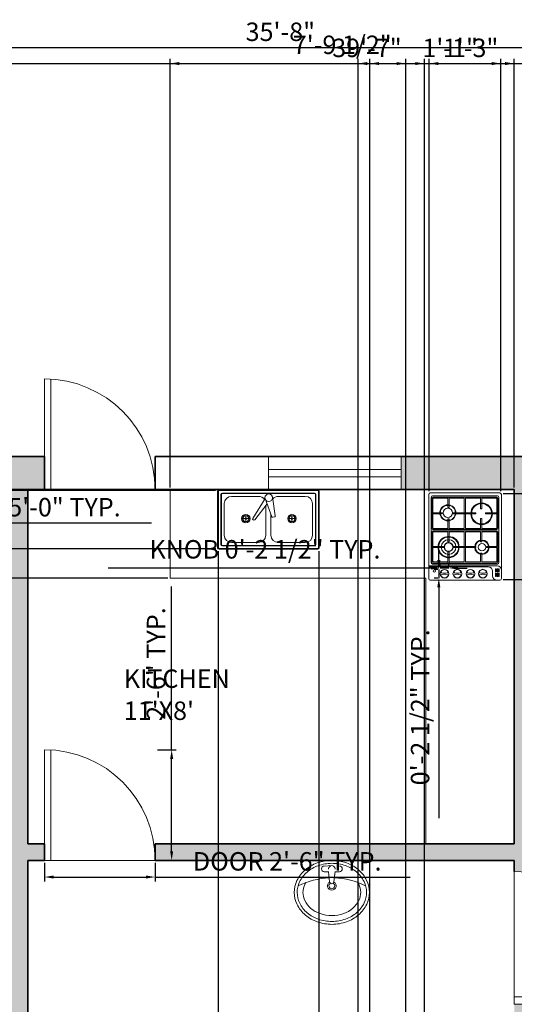
# Model space of a CAD drawing. Units: inches. Extents: x 2923 to 3500, y 1684 to 2381.
# Tile 11 of 12: x 3112 to 3247, y 2114 to 2381. Entities that reach past the tile are written whole.
import ezdxf

# ---------------------------------------------------------------- set-up
doc = ezdxf.new("R2010")
doc.units = ezdxf.units.IN
for name, color, linetype, lineweight in [('A-ANNO-DIMS', 2, 'Continuous', 18), ('A-AREA-IDEN', 7, 'Continuous', 18), ('A-DOOR', 3, 'Continuous', 18), ('A-EQPM', 8, 'Continuous', 18), ('A-FLOR-CASE', 7, 'Continuous', 20), ('A-FLOR-FIXT', 8, 'Continuous', 18), ('A-GLAZ', 4, 'Continuous', 18), ('A-WALL', 7, 'Continuous', 35), ('A-WALL-PATT', 9, 'Continuous', 13)]:
    doc.layers.add(name, color=color, linetype=linetype, lineweight=lineweight)
doc.styles.get("Standard").update_dxf_attribs({"font": 'txt', "height": 5})
doc.dimstyles.new('ISO-25', dxfattribs={"dimtxt": 5, "dimasz": 2.5, "dimexe": 1.25, "dimexo": 0.625, "dimtad": 1, "dimlunit": 3, "dimtxsty": 'Standard', "dimcen": 2.5, "dimadec": 0, "dimazin": 0, "dimtfac": 1, "dimtmove": 0, "dimatfit": 3, "dimfxl": 1, "dimarcsym": 0})

# ---------------------------------------------------------------- blocks, each defined once
blk = doc.blocks.new('*D2')
at = {"layer": 'A-ANNO-DIMS', "color": 0, "lineweight": -2, "transparency": 16777216}
for p, q in [((2969.23, 2263.03), (2969.23, 2374.52)), ((2971.73, 2373.27), (3394.73, 2373.27)), ((3397.23, 2263.03), (3397.23, 2374.52))]:
    blk.add_line(p, q, dxfattribs=at)
at = {"layer": 'A-ANNO-DIMS', "color": 0, "transparency": 16777216}
for points in [[(2971.73, 2373.69), (2971.73, 2372.86), (2969.23, 2373.27)], [(3394.73, 2373.69), (3394.73, 2372.86), (3397.23, 2373.27)]]:
    blk.add_solid(points, dxfattribs=at)
at = {"layer": 'Defpoints', "color": 0, "transparency": 16777216}
for p in [(3397.23, 2373.27), (2969.23, 2262.41), (3397.23, 2262.41)]:
    blk.add_point(p, dxfattribs=at)
at = {"layer": 'A-ANNO-DIMS', "color": 0, "transparency": 16777216, "insert": (3183.23, 2376.87), "char_height": 5, "attachment_point": 5}
blk.add_mtext('35\'-8"', dxfattribs=at)
blk = doc.blocks.new('DOOR-SINGLE-36IN')
for p, q in [((36, 36), (0, 36)), ((34, 0.06), (34, 36)), ((36, 0), (36, 36))]:
    blk.add_line(p, q)
blk.add_arc((36, 36), 36, 180, 270)
blk = doc.blocks.new('DOOR-SINGLE-30IN')
for p, q in [((0, 30), (0, 0)), ((1.67, 29.95), (1.67, 0)), ((0, 0), (30, 0))]:
    blk.add_line(p, q)
blk.add_arc((0, 0), 30, 0, 90)
blk = doc.blocks.new('WINDOW-36IN')
for p, q in [((36, 9), (0, 9)), ((0, 9), (0, 0)), ((36, 0), (36, 9)), ((36, 5.5), (0, 5.5)), ((36, 3.5), (0, 3.5)), ((0, 0), (36, 0))]:
    blk.add_line(p, q)
blk = doc.blocks.new('RANGE-CONTROL-KNOB')
blk.add_circle((1.19, 1.19), 1.19)
for centre, radius, start, end in [((0.4, 1.64), 0.197, 150.2471, 261.5797), ((0.4, 0.73), 0.197, 98.4203, 209.7529), ((1.19, 1.19), 1.11, 29.7529, 150.2471), ((1.19, 1.19), 1.11, 209.7529, 330.2471), ((1.19, 4.76), 3.42, 256.1268, 283.8732), ((1.19, -2.39), 3.42, 76.1268, 103.8732), ((1.98, 1.64), 0.197, 278.4203, 29.7529), ((1.98, 0.73), 0.197, 330.2471, 81.5797)]:
    blk.add_arc(centre, radius, start, end)
blk = doc.blocks.new('*D21')
at = {"layer": 'A-ANNO-DIMS', "color": 0, "lineweight": -2, "transparency": 16777216}
for p, q in [((3014.23, 2252.78), (3014.23, 2243.16)), ((3074.23, 2252.78), (3074.23, 2243.16)), ((3016.73, 2244.41), (3071.73, 2244.41)), ((3074.23, 2244.41), (3148.22, 2244.41))]:
    blk.add_line(p, q, dxfattribs=at)
at = {"layer": 'A-ANNO-DIMS', "color": 0, "transparency": 16777216}
for points in [[(3016.73, 2244.82), (3016.73, 2243.99), (3014.23, 2244.41)], [(3071.73, 2244.82), (3071.73, 2243.99), (3074.23, 2244.41)]]:
    blk.add_solid(points, dxfattribs=at)
at = {"layer": 'Defpoints', "color": 0, "transparency": 16777216}
for p in [(3014.23, 2253.41), (3074.23, 2253.41), (3074.23, 2244.41)]:
    blk.add_point(p, dxfattribs=at)
at = {"layer": 'A-ANNO-DIMS', "color": 0, "transparency": 16777216, "insert": (3112.47, 2248.01), "char_height": 5, "attachment_point": 5}
blk.add_mtext('SLIDER 5\'-0" TYP.', dxfattribs=at)
blk = doc.blocks.new('*D27')
at = {"layer": 'A-ANNO-DIMS', "color": 0, "lineweight": -2, "transparency": 16777216}
for p, q in [((3119.23, 2152.28), (3119.23, 2147.16)), ((3149.23, 2152.28), (3149.23, 2147.16)), ((3121.73, 2148.41), (3146.73, 2148.41)), ((3149.23, 2148.41), (3218.46, 2148.41))]:
    blk.add_line(p, q, dxfattribs=at)
at = {"layer": 'A-ANNO-DIMS', "color": 0, "transparency": 16777216}
for points in [[(3121.73, 2148.82), (3121.73, 2147.99), (3119.23, 2148.41)], [(3146.73, 2148.82), (3146.73, 2147.99), (3149.23, 2148.41)]]:
    blk.add_solid(points, dxfattribs=at)
at = {"layer": 'Defpoints', "color": 0, "transparency": 16777216}
for p in [(3119.23, 2152.91), (3149.23, 2152.91), (3149.23, 2148.41)]:
    blk.add_point(p, dxfattribs=at)
at = {"layer": 'A-ANNO-DIMS', "color": 0, "transparency": 16777216, "insert": (3185.09, 2152.01), "char_height": 5, "attachment_point": 5}
blk.add_mtext('DOOR 2\'-6" TYP.', dxfattribs=at)
blk = doc.blocks.new('*D28')
at = {"layer": 'A-ANNO-DIMS', "color": 0, "lineweight": -2, "transparency": 16777216}
for p, q in [((3153.73, 2182.91), (3153.73, 2227.13)), ((3149.85, 2182.91), (3154.98, 2182.91)), ((3153.73, 2155.41), (3153.73, 2180.41)), ((3149.85, 2152.91), (3154.98, 2152.91))]:
    blk.add_line(p, q, dxfattribs=at)
at = {"layer": 'A-ANNO-DIMS', "color": 0, "transparency": 16777216}
for points in [[(3153.31, 2180.41), (3154.15, 2180.41), (3153.73, 2182.91)], [(3153.31, 2155.41), (3154.15, 2155.41), (3153.73, 2152.91)]]:
    blk.add_solid(points, dxfattribs=at)
at = {"layer": 'Defpoints', "color": 0, "transparency": 16777216}
for p in [(3149.23, 2182.91), (3153.73, 2182.91), (3149.23, 2152.91)]:
    blk.add_point(p, dxfattribs=at)
at = {"layer": 'A-ANNO-DIMS', "color": 0, "transparency": 16777216, "insert": (3150.13, 2206.27), "char_height": 5, "attachment_point": 5, "rotation": 90}
blk.add_mtext('2\'-6" TYP.', dxfattribs=at)
blk = doc.blocks.new('*D43')
at = {"layer": 'A-ANNO-DIMS', "color": 0, "lineweight": -2, "transparency": 16777216}
for p, q in [((3224.09, 2232.16), (3136.53, 2232.16)), ((3226.59, 2232.43), (3226.59, 2233.41)), ((3228.96, 2232.16), (3226.59, 2232.16)), ((3228.96, 2232.43), (3228.96, 2233.41)), ((3231.46, 2232.16), (3233.96, 2232.16))]:
    blk.add_line(p, q, dxfattribs=at)
at = {"layer": 'A-ANNO-DIMS', "color": 0, "transparency": 16777216}
for points in [[(3224.09, 2232.58), (3224.09, 2231.74), (3226.59, 2232.16)], [(3231.46, 2232.58), (3231.46, 2231.74), (3228.96, 2232.16)]]:
    blk.add_solid(points, dxfattribs=at)
at = {"layer": 'Defpoints', "color": 0, "transparency": 16777216}
for p in [(3226.59, 2232.16), (3226.59, 2231.8), (3228.96, 2231.8)]:
    blk.add_point(p, dxfattribs=at)
at = {"layer": 'A-ANNO-DIMS', "color": 0, "transparency": 16777216, "insert": (3179.06, 2236.59), "char_height": 5, "attachment_point": 5}
blk.add_mtext('KNOB 0\'-2 1/2" TYP.', dxfattribs=at)
blk = doc.blocks.new('*D44')
at = {"layer": 'A-ANNO-DIMS', "color": 0, "lineweight": -2, "transparency": 16777216}
for p, q in [((3226.23, 2234.3), (3226.23, 2236.8)), ((3225.96, 2231.8), (3224.98, 2231.8)), ((3226.23, 2231.8), (3226.23, 2229.43)), ((3225.96, 2229.43), (3224.98, 2229.43)), ((3226.23, 2226.93), (3226.23, 2164.37))]:
    blk.add_line(p, q, dxfattribs=at)
at = {"layer": 'A-ANNO-DIMS', "color": 0, "transparency": 16777216}
for points in [[(3225.82, 2234.3), (3226.65, 2234.3), (3226.23, 2231.8)], [(3225.82, 2226.93), (3226.65, 2226.93), (3226.23, 2229.43)]]:
    blk.add_solid(points, dxfattribs=at)
at = {"layer": 'Defpoints', "color": 0, "transparency": 16777216}
for p in [(3226.59, 2231.8), (3226.23, 2229.43), (3226.59, 2229.43)]:
    blk.add_point(p, dxfattribs=at)
at = {"layer": 'A-ANNO-DIMS', "color": 0, "transparency": 16777216, "insert": (3221.8, 2194.4), "char_height": 5, "attachment_point": 5, "rotation": 90}
blk.add_mtext('0\'-2 1/2" TYP.', dxfattribs=at)
blk = doc.blocks.new('*D49')
at = {"layer": 'A-ANNO-DIMS', "color": 0, "lineweight": -2, "transparency": 16777216}
for p, q in [((2969.23, 2263.03), (2969.23, 2370.16)), ((3444.23, 2110.03), (3444.23, 2370.16)), ((2971.73, 2368.91), (3441.73, 2368.91))]:
    blk.add_line(p, q, dxfattribs=at)
at = {"layer": 'A-ANNO-DIMS', "color": 0, "transparency": 16777216}
for points in [[(2971.73, 2369.32), (2971.73, 2368.49), (2969.23, 2368.91)], [(3441.73, 2369.32), (3441.73, 2368.49), (3444.23, 2368.91)]]:
    blk.add_solid(points, dxfattribs=at)
at = {"layer": 'Defpoints', "color": 0, "transparency": 16777216}
for p in [(3444.23, 2368.91), (2969.23, 2262.41), (3444.23, 2109.41)]:
    blk.add_point(p, dxfattribs=at)
at = {"layer": 'A-ANNO-DIMS', "color": 0, "transparency": 16777216, "insert": (3206.73, 2372.51), "char_height": 5, "attachment_point": 5}
blk.add_mtext('39\'-7"', dxfattribs=at)
blk = doc.blocks.new('*D52')
at = {"layer": 'A-ANNO-DIMS', "color": 0, "lineweight": -2, "transparency": 16777216}
for p, q in [((3152.68, 2253.41), (2933.48, 2253.41)), ((2934.73, 2250.91), (2934.73, 2231.91)), ((3152.68, 2229.41), (2933.48, 2229.41))]:
    blk.add_line(p, q, dxfattribs=at)
at = {"layer": 'A-ANNO-DIMS', "color": 0, "transparency": 16777216}
for points in [[(2934.31, 2250.91), (2935.15, 2250.91), (2934.73, 2253.41)], [(2934.31, 2231.91), (2935.15, 2231.91), (2934.73, 2229.41)]]:
    blk.add_solid(points, dxfattribs=at)
at = {"layer": 'Defpoints', "color": 0, "transparency": 16777216}
for p in [(3153.3, 2253.41), (2934.73, 2229.41), (3153.3, 2229.41)]:
    blk.add_point(p, dxfattribs=at)
at = {"layer": 'A-ANNO-DIMS', "color": 0, "transparency": 16777216, "insert": (2931.13, 2241.41), "char_height": 5, "attachment_point": 5, "rotation": 90}
blk.add_mtext('2\'-0"', dxfattribs=at)
blk = doc.blocks.new('*D53')
at = {"layer": 'A-ANNO-DIMS', "color": 0, "lineweight": -2, "transparency": 16777216}
for p, q in [((3153.3, 2254.03), (3153.3, 2370.16)), ((3246.73, 2254.03), (3246.73, 2370.16)), ((3155.8, 2368.91), (3244.23, 2368.91))]:
    blk.add_line(p, q, dxfattribs=at)
at = {"layer": 'A-ANNO-DIMS', "color": 0, "transparency": 16777216}
for points in [[(3155.8, 2369.32), (3155.8, 2368.49), (3153.3, 2368.91)], [(3244.23, 2369.32), (3244.23, 2368.49), (3246.73, 2368.91)]]:
    blk.add_solid(points, dxfattribs=at)
at = {"layer": 'Defpoints', "color": 0, "transparency": 16777216}
for p in [(3246.73, 2368.91), (3153.3, 2253.41), (3246.73, 2253.41)]:
    blk.add_point(p, dxfattribs=at)
at = {"layer": 'A-ANNO-DIMS', "color": 0, "transparency": 16777216, "insert": (3200.02, 2373.34), "char_height": 5, "attachment_point": 5}
blk.add_mtext('7\'-9 1/2"', dxfattribs=at)
blk = doc.blocks.new('*D54')
at = {"layer": 'A-ANNO-DIMS', "color": 0, "lineweight": -2, "transparency": 16777216}
for p, q in [((3166.32, 2236.75), (3166.32, 1685.66)), ((3193.64, 2236.75), (3193.64, 1685.66)), ((3168.82, 1686.91), (3191.14, 1686.91)), ((3193.64, 1686.91), (3235.49, 1686.91))]:
    blk.add_line(p, q, dxfattribs=at)
at = {"layer": 'A-ANNO-DIMS', "color": 0, "transparency": 16777216}
for points in [[(3168.82, 1687.32), (3168.82, 1686.49), (3166.32, 1686.91)], [(3191.14, 1687.32), (3191.14, 1686.49), (3193.64, 1686.91)]]:
    blk.add_solid(points, dxfattribs=at)
at = {"layer": 'Defpoints', "color": 0, "transparency": 16777216}
for p in [(3166.32, 2237.38), (3193.64, 2237.38), (3193.64, 1686.91)]:
    blk.add_point(p, dxfattribs=at)
at = {"layer": 'A-ANNO-DIMS', "color": 0, "transparency": 16777216, "insert": (3215.82, 1691.34), "char_height": 5, "attachment_point": 5}
blk.add_mtext('2\'-3 1/2"', dxfattribs=at)
blk = doc.blocks.new('*D55')
at = {"layer": 'A-ANNO-DIMS', "color": 0, "lineweight": -2, "transparency": 16777216}
for p, q in [((2934.73, 2253.17), (2934.73, 2275.73)), ((3165.61, 2253.17), (2933.48, 2253.17)), ((2934.73, 2239.88), (2934.73, 2250.67)), ((3165.69, 2237.38), (2933.48, 2237.38))]:
    blk.add_line(p, q, dxfattribs=at)
at = {"layer": 'A-ANNO-DIMS', "color": 0, "transparency": 16777216}
for points in [[(2934.31, 2250.67), (2935.15, 2250.67), (2934.73, 2253.17)], [(2934.31, 2239.88), (2935.15, 2239.88), (2934.73, 2237.38)]]:
    blk.add_solid(points, dxfattribs=at)
at = {"layer": 'Defpoints', "color": 0, "transparency": 16777216}
for p in [(2934.73, 2253.17), (3166.23, 2253.17), (3166.32, 2237.38)]:
    blk.add_point(p, dxfattribs=at)
at = {"layer": 'A-ANNO-DIMS', "color": 0, "transparency": 16777216, "insert": (2931.13, 2265.7), "char_height": 5, "attachment_point": 5, "rotation": 90}
blk.add_mtext('1\'-4"', dxfattribs=at)
blk = doc.blocks.new('*D56')
at = {"layer": 'A-ANNO-DIMS', "color": 0, "lineweight": -2, "transparency": 16777216}
for p, q in [((3223.64, 2253.03), (3223.64, 2370.16)), ((3243.09, 2253.03), (3243.09, 2370.16)), ((3226.14, 2368.91), (3240.59, 2368.91)), ((3243.09, 2368.91), (3283.99, 2368.91))]:
    blk.add_line(p, q, dxfattribs=at)
at = {"layer": 'A-ANNO-DIMS', "color": 0, "transparency": 16777216}
for points in [[(3226.14, 2369.32), (3226.14, 2368.49), (3223.64, 2368.91)], [(3240.59, 2369.32), (3240.59, 2368.49), (3243.09, 2368.91)]]:
    blk.add_solid(points, dxfattribs=at)
at = {"layer": 'Defpoints', "color": 0, "transparency": 16777216}
for p in [(3243.09, 2368.91), (3223.64, 2252.4), (3243.09, 2252.4)]:
    blk.add_point(p, dxfattribs=at)
at = {"layer": 'A-ANNO-DIMS', "color": 0, "transparency": 16777216, "insert": (3264.79, 2373.34), "char_height": 5, "attachment_point": 5}
blk.add_mtext('1\'-7 1/2"', dxfattribs=at)
blk = doc.blocks.new('*D57')
at = {"layer": 'A-ANNO-DIMS', "color": 0, "lineweight": -2, "transparency": 16777216}
for p, q in [((3243.72, 2252.4), (3479.98, 2252.4)), ((3478.73, 2249.9), (3478.73, 2231.51)), ((3243.72, 2229.01), (3479.98, 2229.01)), ((3478.73, 2229.01), (3478.73, 2185.26))]:
    blk.add_line(p, q, dxfattribs=at)
at = {"layer": 'A-ANNO-DIMS', "color": 0, "transparency": 16777216}
for points in [[(3478.31, 2249.9), (3479.15, 2249.9), (3478.73, 2252.4)], [(3478.31, 2231.51), (3479.15, 2231.51), (3478.73, 2229.01)]]:
    blk.add_solid(points, dxfattribs=at)
at = {"layer": 'Defpoints', "color": 0, "transparency": 16777216}
for p in [(3243.09, 2252.4), (3243.09, 2229.01), (3478.73, 2229.01)]:
    blk.add_point(p, dxfattribs=at)
at = {"layer": 'A-ANNO-DIMS', "color": 0, "transparency": 16777216, "insert": (3474.3, 2205.88), "char_height": 5, "attachment_point": 5, "rotation": 90}
blk.add_mtext('1\'-11 1/2"', dxfattribs=at)
blk = doc.blocks.new('*D62')
at = {"layer": 'A-ANNO-DIMS', "color": 0, "lineweight": -2, "transparency": 16777216}
for p, q in [((3204.33, 1920.39), (3204.33, 2370.16)), ((3217.26, 1920.39), (3217.26, 2370.16)), ((3206.83, 2368.91), (3214.76, 2368.91)), ((3217.26, 2368.91), (3238.87, 2368.91))]:
    blk.add_line(p, q, dxfattribs=at)
at = {"layer": 'A-ANNO-DIMS', "color": 0, "transparency": 16777216}
for points in [[(3206.83, 2369.32), (3206.83, 2368.49), (3204.33, 2368.91)], [(3214.76, 2369.32), (3214.76, 2368.49), (3217.26, 2368.91)]]:
    blk.add_solid(points, dxfattribs=at)
at = {"layer": 'Defpoints', "color": 0, "transparency": 16777216}
for p in [(3217.26, 2368.91), (3204.33, 1919.77), (3217.26, 1919.77)]:
    blk.add_point(p, dxfattribs=at)
at = {"layer": 'A-ANNO-DIMS', "color": 0, "transparency": 16777216, "insert": (3229.31, 2372.51), "char_height": 5, "attachment_point": 5}
blk.add_mtext('1\'-1"', dxfattribs=at)
blk = doc.blocks.new('*D66')
at = {"layer": 'A-ANNO-DIMS', "color": 0, "lineweight": -2, "transparency": 16777216}
for p, q in [((3207.52, 1946.69), (3207.52, 2370.16)), ((3222.33, 1946.69), (3222.33, 2370.16)), ((3210.02, 2368.91), (3219.83, 2368.91)), ((3222.33, 2368.91), (3244.89, 2368.91))]:
    blk.add_line(p, q, dxfattribs=at)
at = {"layer": 'A-ANNO-DIMS', "color": 0, "transparency": 16777216}
for points in [[(3210.02, 2369.32), (3210.02, 2368.49), (3207.52, 2368.91)], [(3219.83, 2369.32), (3219.83, 2368.49), (3222.33, 2368.91)]]:
    blk.add_solid(points, dxfattribs=at)
at = {"layer": 'Defpoints', "color": 0, "transparency": 16777216}
for p in [(3222.33, 2368.91), (3207.52, 1946.07), (3222.33, 1946.07)]:
    blk.add_point(p, dxfattribs=at)
at = {"layer": 'A-ANNO-DIMS', "color": 0, "transparency": 16777216, "insert": (3234.86, 2372.51), "char_height": 5, "attachment_point": 5}
blk.add_mtext('1\'-3"', dxfattribs=at)

msp = doc.modelspace()

# ---------------------------------------------------------------- hatches: boundary and pattern name
at = {"layer": 'A-WALL-PATT'}
h = msp.add_hatch(color=256, dxfattribs=at)
h.dxf.hatch_style = 1
h.paths.add_polyline_path([(3014.23, 2262.406), (2969.23, 2262.406), (2969.23, 2201.5), (2978.23, 2201.5), (2978.23, 2213.699), (2978.23, 2253.406), (3014.23, 2253.406)])
h.paths.add_polyline_path([(3119.23, 2262.406), (3074.23, 2262.406), (3074.23, 2253.406), (3110.23, 2253.406), (3110.23, 2109.406), (3105.73, 2109.406), (3105.73, 2104.906), (3114.73, 2104.906), (3114.73, 2152.906), (3119.23, 2152.906), (3119.23, 2157.406), (3114.73, 2157.406), (3114.73, 2253.406), (3119.23, 2253.406)])
h.paths.add_polyline_path([(3179.98, 2262.406), (3149.23, 2262.406), (3149.23, 2253.406), (3179.98, 2253.406)], flags=0)
h.paths.add_polyline_path([(3295.73, 2262.406), (3215.98, 2262.406), (3215.98, 2253.406), (3246.73, 2253.406), (3246.73, 2157.406), (3149.23, 2157.406), (3149.23, 2152.906), (3246.73, 2152.906), (3246.73, 2149.906), (3251.23, 2149.906), (3251.23, 2253.406), (3295.73, 2253.406)])
h.paths.add_polyline_path([(3397.23, 2262.406), (3343.73, 2262.406), (3343.73, 2253.406), (3349.929, 2253.406), (3388.23, 2253.406), (3388.23, 2199.406), (3397.23, 2199.406)])
h.paths.add_polyline_path([(3369.935, 2334.406), (3264.935, 2334.406), (3264.935, 2262.406), (3269.435, 2262.406), (3269.435, 2329.906), (3365.435, 2329.906), (3365.435, 2262.406), (3369.935, 2262.406)])
h.paths.add_polyline_path([(3096.73, 2334.406), (2991.73, 2334.406), (2991.73, 2262.406), (2996.23, 2262.406), (2996.23, 2329.906), (3092.23, 2329.906), (3092.23, 2262.406), (3096.73, 2262.406)])
h.paths.add_polyline_path([(3397.23, 2163.406), (3388.23, 2163.406), (3388.23, 2109.406), (3251.23, 2109.406), (3251.23, 2113.906), (3246.73, 2113.906), (3246.73, 2092.906), (3251.23, 2092.906), (3251.23, 2104.906), (3435.23, 2104.906), (3435.23, 2080.906), (3444.23, 2080.906), (3444.23, 2109.406), (3397.23, 2109.406)])
h.paths.add_polyline_path([(3444.23, 2044.906), (3435.23, 2044.906), (3435.23, 2020.906), (3251.23, 2020.906), (3251.23, 2032.906), (3246.73, 2032.906), (3246.73, 2016.406), (3251.23, 2016.406), (3287.73, 2016.406), (3287.73, 1968.406), (3287.23, 1968.406), (3287.23, 1963.906), (3296.73, 1963.906), (3296.73, 1968.406), (3292.23, 1968.406), (3292.23, 2016.406), (3388.23, 2016.406), (3388.23, 2004.398), (3397.23, 2004.398), (3397.23, 2016.406), (3444.23, 2016.406)])
h.paths.add_polyline_path([(3397.23, 1980.398), (3388.23, 1980.398), (3388.23, 1979.998), (3388.23, 1969.828), (3388.23, 1968.406), (3326.73, 1968.406), (3326.73, 1963.906), (3388.23, 1963.906), (3388.23, 1913.156), (3397.23, 1913.156)])
h.paths.add_polyline_path([(3251.23, 1968.406), (3150.73, 1968.406), (3150.73, 1963.906), (3246.73, 1963.906), (3246.73, 1826.406), (3230.98, 1826.406), (3230.98, 1817.406), (3251.23, 1817.406), (3251.23, 1963.906)])
h.paths.add_polyline_path([(3114.73, 1968.406), (3105.73, 1968.406), (3105.73, 1963.906), (3110.23, 1963.906), (3110.23, 1817.406), (3119.23, 1817.406), (3119.23, 1826.406), (3114.73, 1826.406)])
h.paths.add_polyline_path([(3069.73, 1968.406), (3066.73, 1968.406), (3066.73, 1972.906), (3062.23, 1972.906), (3062.23, 1968.406), (2978.23, 1968.406), (2978.23, 1989.406), (2969.23, 1989.406), (2969.23, 1912.505), (2978.23, 1912.505), (2978.23, 1925.355), (2978.23, 1963.906), (3069.73, 1963.906)])
h.paths.add_polyline_path([(3066.73, 2104.906), (3069.73, 2104.906), (3069.73, 2109.406), (3057.73, 2109.406), (3057.73, 2104.906), (3062.23, 2104.906), (3062.23, 2038.906), (2978.23, 2038.906), (2978.23, 2059.906), (2969.23, 2059.906), (2969.23, 2013.406), (2978.23, 2013.406), (2978.23, 2034.406), (3062.23, 2034.406), (3062.23, 2002.906), (3066.73, 2002.906)])
h.paths.add_polyline_path([(3027.73, 2109.406), (2978.23, 2109.406), (2978.23, 2165.5), (2969.23, 2165.5), (2969.23, 2083.906), (2978.23, 2083.906), (2978.23, 2104.906), (3027.73, 2104.906)])
h.paths.add_polyline_path([(2978.23, 1876.505), (2969.23, 1876.505), (2969.23, 1817.406), (3014.23, 1817.406), (3014.23, 1826.406), (2978.23, 1826.406)])
h.paths.add_polyline_path([(2996.23, 1817.406), (2991.73, 1817.406), (2991.73, 1745.406), (3096.73, 1745.406), (3096.73, 1817.406), (3092.23, 1817.406), (3092.23, 1749.906), (2996.23, 1749.906)])
h.paths.add_polyline_path([(3289.73, 1826.406), (3251.23, 1826.406), (3251.23, 1817.406), (3289.73, 1817.406)])
h.paths.add_polyline_path([(3397.23, 1877.156), (3388.23, 1877.156), (3388.23, 1864.957), (3388.23, 1826.406), (3349.73, 1826.406), (3349.73, 1817.406), (3397.23, 1817.406)])
h.paths.add_polyline_path([(3374.267, 1817.406), (3369.767, 1817.406), (3369.767, 1749.906), (3273.767, 1749.906), (3273.767, 1817.406), (3269.267, 1817.406), (3269.267, 1745.406), (3374.267, 1745.406)])

# ---------------------------------------------------------------- linework, layer by layer
at = {"layer": 'A-EQPM'}
for p, q in [((3223.525, 2252.123), (3223.525, 2229.288)), ((3242.816, 2252.516), (3223.919, 2252.516)), ((3224.127, 2251.323), (3224.127, 2233.647)), ((3224.338, 2242.879), (3224.338, 2251.107)), ((3242.125, 2251.717), (3224.521, 2251.717)), ((3224.613, 2251.383), (3241.997, 2251.383)), ((3224.653, 2247.151), (3224.653, 2251.068)), ((3224.653, 2251.068), (3228.704, 2251.068)), ((3228.704, 2251.383), (3228.704, 2248.555)), ((3229.018, 2251.383), (3229.018, 2248.555)), ((3229.018, 2251.068), (3233.069, 2251.068)), ((3233.148, 2250.989), (3233.148, 2247.151)), ((3233.463, 2250.989), (3233.463, 2247.151)), ((3233.542, 2251.068), (3237.592, 2251.068)), ((3237.592, 2251.383), (3237.592, 2248.172)), ((3237.907, 2251.383), (3237.907, 2248.172)), ((3237.907, 2251.068), (3241.958, 2251.068)), ((3241.958, 2251.068), (3241.958, 2247.151)), ((3242.273, 2251.107), (3242.273, 2242.879)), ((3242.518, 2233.647), (3242.518, 2251.323)), ((3243.21, 2229.288), (3243.21, 2252.123)), ((3229.018, 2248.555), (3228.704, 2248.555)), ((3237.907, 2248.172), (3237.592, 2248.172)), ((3224.338, 2247.151), (3227.166, 2247.151)), ((3224.338, 2246.836), (3227.166, 2246.836)), ((3224.653, 2242.918), (3224.653, 2246.836)), ((3227.166, 2247.151), (3227.166, 2246.836)), ((3229.018, 2245.538), (3228.704, 2245.538)), ((3228.704, 2242.603), (3228.704, 2245.538)), ((3229.018, 2242.603), (3229.018, 2245.538)), ((3230.137, 2246.993), (3230.137, 2247.151)), ((3230.137, 2247.151), (3236.292, 2247.151)), ((3230.137, 2246.993), (3230.137, 2246.836)), ((3230.137, 2246.836), (3236.292, 2246.836)), ((3233.148, 2246.836), (3233.148, 2242.997)), ((3233.463, 2246.836), (3233.463, 2242.997)), ((3236.292, 2247.151), (3236.292, 2246.836)), ((3237.592, 2245.623), (3237.907, 2245.623)), ((3237.592, 2242.603), (3237.592, 2245.623)), ((3237.907, 2242.603), (3237.907, 2245.623)), ((3238.924, 2246.836), (3238.924, 2247.151)), ((3242.273, 2247.151), (3238.924, 2247.151)), ((3242.273, 2246.836), (3238.924, 2246.836)), ((3241.958, 2246.836), (3241.958, 2242.918)), ((3224.338, 2233.767), (3224.338, 2241.995)), ((3241.997, 2242.603), (3224.613, 2242.603)), ((3224.613, 2242.271), (3241.997, 2242.271)), ((3228.704, 2242.918), (3224.653, 2242.918)), ((3224.653, 2241.956), (3228.704, 2241.956)), ((3224.653, 2238.038), (3224.653, 2241.956)), ((3228.704, 2242.271), (3228.704, 2239.223)), ((3233.069, 2242.918), (3229.018, 2242.918)), ((3229.018, 2242.271), (3229.018, 2239.223)), ((3229.018, 2241.956), (3233.069, 2241.956)), ((3237.592, 2242.918), (3233.542, 2242.918)), ((3233.542, 2241.956), (3237.592, 2241.956)), ((3237.592, 2241.956), (3237.592, 2239.25)), ((3241.958, 2242.918), (3237.907, 2242.918)), ((3237.907, 2241.956), (3241.958, 2241.956)), ((3237.907, 2241.956), (3237.907, 2239.25)), ((3241.958, 2241.956), (3241.958, 2238.038)), ((3242.273, 2241.995), (3242.273, 2233.767)), ((3229.018, 2239.223), (3228.704, 2239.223)), ((3233.148, 2241.877), (3233.148, 2238.038)), ((3233.463, 2241.877), (3233.463, 2238.038)), ((3237.907, 2239.25), (3237.592, 2239.25)), ((3224.338, 2238.038), (3227.548, 2238.038)), ((3224.338, 2237.723), (3227.548, 2237.723)), ((3224.653, 2233.806), (3224.653, 2237.723)), ((3227.548, 2238.038), (3227.548, 2237.723)), ((3230.264, 2238.038), (3230.264, 2237.723)), ((3236.25, 2238.038), (3230.264, 2238.038)), ((3236.25, 2237.723), (3230.264, 2237.723)), ((3233.148, 2237.723), (3233.148, 2233.885)), ((3233.463, 2237.723), (3233.463, 2233.885)), ((3236.25, 2237.881), (3236.25, 2238.038)), ((3236.25, 2237.881), (3236.25, 2237.723)), ((3239.136, 2238.038), (3239.136, 2237.723)), ((3241.958, 2238.038), (3239.136, 2238.038)), ((3241.958, 2237.723), (3239.136, 2237.723)), ((3241.958, 2237.723), (3241.958, 2233.806)), ((3228.704, 2236.53), (3229.018, 2236.53)), ((3228.704, 2233.491), (3228.704, 2236.53)), ((3229.018, 2233.491), (3229.018, 2236.53)), ((3237.907, 2236.233), (3237.592, 2236.233)), ((3237.592, 2233.806), (3237.592, 2236.233)), ((3237.907, 2233.806), (3237.907, 2236.233)), ((3223.525, 2232.784), (3223.525, 2232.485)), ((3242.029, 2232.784), (3223.525, 2232.784)), ((3223.525, 2232.485), (3239.658, 2232.485)), ((3224.521, 2233.254), (3242.125, 2233.254)), ((3241.997, 2233.491), (3224.613, 2233.491)), ((3228.704, 2233.806), (3224.653, 2233.806)), ((3233.069, 2233.806), (3229.018, 2233.806)), ((3237.592, 2233.806), (3233.542, 2233.806)), ((3241.958, 2233.806), (3237.907, 2233.806)), ((3240.839, 2231.304), (3240.839, 2230.076)), ((3241.631, 2231.149), (3241.631, 2231.93)), ((3241.69, 2231.989), (3241.717, 2231.989)), ((3241.776, 2231.93), (3241.776, 2231.149)), ((3242.067, 2231.149), (3242.067, 2231.93)), ((3242.126, 2231.989), (3242.153, 2231.989)), ((3242.212, 2231.93), (3242.212, 2231.149)), ((3242.478, 2231.149), (3242.478, 2231.93)), ((3242.537, 2231.989), (3242.564, 2231.989)), ((3242.623, 2231.93), (3242.623, 2231.149)), ((3243.21, 2229.288), (3243.21, 2231.602)), ((3223.919, 2228.894), (3242.816, 2228.894)), ((3241.631, 2229.941), (3241.631, 2230.722)), ((3241.717, 2231.09), (3241.69, 2231.09)), ((3241.69, 2230.781), (3241.717, 2230.781)), ((3241.717, 2229.882), (3241.69, 2229.882)), ((3241.776, 2230.722), (3241.776, 2229.941)), ((3242.02, 2228.894), (3242.816, 2228.894)), ((3242.067, 2229.941), (3242.067, 2230.722)), ((3242.153, 2231.09), (3242.126, 2231.09)), ((3242.126, 2230.781), (3242.153, 2230.781)), ((3242.153, 2229.882), (3242.126, 2229.882)), ((3242.212, 2230.722), (3242.212, 2229.941)), ((3242.478, 2229.941), (3242.478, 2230.722)), ((3242.564, 2231.09), (3242.537, 2231.09)), ((3242.537, 2230.781), (3242.564, 2230.781)), ((3242.564, 2229.882), (3242.537, 2229.882)), ((3242.623, 2230.722), (3242.623, 2229.941))]:
    msp.add_line(p, q, dxfattribs=at)
for centre, radius in [((3228.69, 2247.128), 2.185), ((3228.69, 2247.128), 2.027), ((3228.69, 2247.128), 1.24), ((3237.857, 2246.874), 2.941), ((3237.857, 2246.874), 2.744), ((3228.884, 2237.842), 2.875), ((3228.884, 2237.842), 2.717), ((3228.884, 2237.842), 2.009), ((3237.947, 2237.802), 1.955), ((3237.947, 2237.802), 1.798), ((3228.884, 2237.842), 1.221), ((3228.884, 2237.842), 1.142), ((3237.947, 2237.802), 1.01), ((3225.026, 2231.363), 0.285)]:
    msp.add_circle(centre, radius, dxfattribs=at)
for centre, radius, start, end in [((3223.919, 2252.123), 0.394, 90, 180), ((3224.521, 2251.323), 0.394, 90, 180), ((3224.613, 2251.107), 0.276, 90, 180), ((3233.069, 2250.989), 0.0787, 0, 90), ((3233.542, 2250.989), 0.0787, 90, 180), ((3241.997, 2251.107), 0.276, 0, 90), ((3242.125, 2251.323), 0.394, 0, 90), ((3242.816, 2252.123), 0.394, 0, 90), ((3224.613, 2242.879), 0.276, 180, 270), ((3224.613, 2241.995), 0.276, 90, 180), ((3233.069, 2242.997), 0.0787, 270, 0), ((3233.069, 2241.877), 0.0787, 0, 90), ((3233.542, 2242.997), 0.0787, 180, 270), ((3233.542, 2241.877), 0.0787, 90, 180), ((3241.997, 2242.879), 0.276, 270, 360), ((3241.997, 2241.995), 0.276, 0, 90), ((3233.069, 2233.885), 0.0787, 270, 0), ((3233.542, 2233.885), 0.0787, 180, 270), ((3224.521, 2233.647), 0.394, 180, 270), ((3224.613, 2233.767), 0.276, 180, 270), ((3239.658, 2231.304), 1.181, 0, 90), ((3241.69, 2231.93), 0.0591, 90, 180), ((3241.717, 2231.93), 0.0591, 0, 90), ((3241.997, 2233.767), 0.276, 270, 0), ((3242.029, 2231.602), 1.181, 0, 90), ((3242.126, 2231.93), 0.0591, 90, 180), ((3242.125, 2233.647), 0.394, 270, 0), ((3242.153, 2231.93), 0.0591, 0, 90), ((3242.537, 2231.93), 0.0591, 90, 180), ((3242.564, 2231.93), 0.0591, 0, 90), ((3223.919, 2229.288), 0.394, 180, 270), ((3242.02, 2230.076), 1.181, 180, 270), ((3241.69, 2231.149), 0.0591, 180, 270), ((3241.69, 2230.722), 0.0591, 90, 180), ((3241.69, 2229.941), 0.0591, 180, 270), ((3241.717, 2231.149), 0.0591, 270, 0), ((3241.717, 2230.722), 0.0591, 0, 90), ((3241.717, 2229.941), 0.0591, 270, 360), ((3242.126, 2231.149), 0.0591, 180, 270), ((3242.126, 2230.722), 0.0591, 90, 180), ((3242.126, 2229.941), 0.0591, 180, 270), ((3242.153, 2231.149), 0.0591, 270, 0), ((3242.153, 2230.722), 0.0591, 0, 90), ((3242.153, 2229.941), 0.0591, 270, 360), ((3242.537, 2231.149), 0.0591, 180, 270), ((3242.537, 2230.722), 0.0591, 90, 180), ((3242.537, 2229.941), 0.0591, 180, 270), ((3242.564, 2231.149), 0.0591, 270, 0), ((3242.564, 2230.722), 0.0591, 0, 90), ((3242.564, 2229.941), 0.0591, 270, 360), ((3242.816, 2229.288), 0.394, 270, 0), ((3242.816, 2229.288), 0.394, 270, 0)]:
    msp.add_arc(centre, radius, start, end, dxfattribs=at)
at = {"layer": 'A-FLOR-CASE'}
for p, q in [((3153.303, 2229.406), (3153.303, 2253.406)), ((3153.303, 2229.406), (3222.73, 2229.406)), ((3222.73, 2157.406), (3222.73, 2229.406))]:
    msp.add_line(p, q, dxfattribs=at)
at = {"layer": 'A-FLOR-FIXT'}
for p, q in [((3166.2, 2253.013), (3166.2, 2237.658)), ((3166.397, 2253.013), (3166.397, 2237.658)), ((3193.366, 2253.406), (3166.594, 2253.406)), ((3193.366, 2253.209), (3166.594, 2253.209)), ((3193.562, 2237.658), (3193.562, 2253.013)), ((3193.759, 2237.658), (3193.759, 2253.013)), ((3167.106, 2252.107), (3167.106, 2238.564)), ((3167.224, 2252.107), (3167.224, 2238.564)), ((3192.46, 2252.501), (3167.5, 2252.501)), ((3192.46, 2252.383), (3167.5, 2252.383)), ((3177.303, 2251.595), (3169.98, 2251.595)), ((3179.082, 2250.968), (3175.733, 2245.622)), ((3179.082, 2250.968), (3180.937, 2246.045)), ((3181.865, 2246.285), (3181.071, 2251.477)), ((3189.98, 2251.595), (3182.657, 2251.595)), ((3192.736, 2238.564), (3192.736, 2252.107)), ((3192.854, 2238.564), (3192.854, 2252.107)), ((3168.011, 2249.627), (3168.011, 2241.044)), ((3179.607, 2249.576), (3176.274, 2245.245)), ((3179.271, 2241.044), (3179.271, 2249.139)), ((3191.948, 2241.044), (3191.948, 2249.627)), ((3173.656, 2245.547), (3173.065, 2245.547)), ((3173.859, 2245.751), (3173.859, 2246.341)), ((3173.859, 2245.343), (3173.859, 2244.753)), ((3174.063, 2245.547), (3174.654, 2245.547)), ((3175.838, 2245.183), (3175.813, 2245.202)), ((3180.688, 2246.706), (3180.688, 2241.044)), ((3181.17, 2245.924), (3181.719, 2246.064)), ((3186.173, 2245.547), (3185.583, 2245.547)), ((3186.377, 2245.751), (3186.377, 2246.341)), ((3186.377, 2245.343), (3186.377, 2244.753)), ((3186.581, 2245.547), (3187.171, 2245.547)), ((3166.594, 2237.461), (3193.366, 2237.461)), ((3166.594, 2237.265), (3193.366, 2237.265)), ((3167.5, 2238.288), (3192.46, 2238.288)), ((3167.5, 2238.17), (3192.46, 2238.17)), ((3169.98, 2239.076), (3177.303, 2239.076)), ((3182.657, 2239.076), (3189.98, 2239.076)), ((3195.156, 2151.371), (3197.203, 2151.496)), ((3195.161, 2149.836), (3196.4, 2149.84)), ((3196.305, 2149.856), (3196.61, 2147.101)), ((3198.066, 2149.862), (3197.781, 2147.105)), ((3199.256, 2149.85), (3198.017, 2149.845))]:
    msp.add_line(p, q, dxfattribs=at)
for centre, radius in [((3180.076, 2251.223), 1.026), ((3173.859, 2245.547), 1.162), ((3173.859, 2245.547), 1.099), ((3173.859, 2245.547), 0.83), ((3173.859, 2245.547), 0.794), ((3173.859, 2245.547), 0.204), ((3173.859, 2245.547), 0.0958), ((3186.377, 2245.547), 1.162), ((3186.377, 2245.547), 1.099), ((3186.377, 2245.547), 0.83), ((3186.377, 2245.547), 0.794), ((3186.377, 2245.547), 0.204), ((3186.377, 2245.547), 0.0958)]:
    msp.add_circle(centre, radius, dxfattribs=at)
for centre, radius, start, end in [((3166.594, 2253.013), 0.394, 90, 180), ((3166.594, 2253.013), 0.197, 90, 180), ((3193.366, 2253.013), 0.394, 0, 90), ((3193.366, 2253.013), 0.197, 0, 90), ((3167.5, 2252.107), 0.394, 90, 180), ((3167.5, 2252.107), 0.276, 90, 180), ((3169.98, 2249.627), 1.968, 90, 180), ((3177.303, 2249.627), 1.968, 34.08644, 90), ((3182.657, 2249.627), 1.968, 90, 139.57501), ((3189.98, 2249.627), 1.968, 0, 90), ((3192.46, 2252.107), 0.394, 0, 90), ((3192.46, 2252.107), 0.276, 0, 90), ((3176, 2245.455), 0.315, 147.93014, 233.63093), ((3176.024, 2245.437), 0.315, 233.63093, 322.41854), ((3181.122, 2246.115), 0.197, 200.64982, 284.32333), ((3181.67, 2246.255), 0.197, 284.32333, 8.69854), ((3169.98, 2241.044), 1.968, 180, 270), ((3177.303, 2241.044), 1.968, 270, 0), ((3182.657, 2241.044), 1.968, 180, 270), ((3189.98, 2241.044), 1.968, 270, 0), ((3166.594, 2237.658), 0.394, 180, 270), ((3166.594, 2237.658), 0.197, 180, 270), ((3167.5, 2238.564), 0.394, 180, 270), ((3167.5, 2238.564), 0.276, 180, 270), ((3192.46, 2238.564), 0.276, 270, 360), ((3192.46, 2238.564), 0.394, 270, 0), ((3193.366, 2237.658), 0.197, 270, 0), ((3193.366, 2237.658), 0.394, 270, 0), ((3196.641, 2142.55), 10.257, 109.58097, 130.54225), ((3196.641, 2142.55), 9.469, 109.58097, 130.54225), ((3197.216, 2140.932), 11.974, 90.19698, 109.58097), ((3197.216, 2140.932), 11.187, 90.19698, 109.58097), ((3195.159, 2150.603), 0.768, 90.19698, 270.19698), ((3197.206, 2150.61), 0.886, 354.08148, 186.31248), ((3197.216, 2140.932), 11.974, 70.81298, 90.19698), ((3197.216, 2140.932), 11.187, 70.81298, 90.19698), ((3199.253, 2150.617), 0.768, 270.19698, 90.19698), ((3197.781, 2142.554), 9.469, 49.85171, 70.81298), ((3197.781, 2142.554), 10.257, 49.85171, 70.81298), ((3195.76, 2143.579), 8.902, 130.54225, 154.20116), ((3195.76, 2143.579), 8.115, 130.54225, 154.20116), ((3198.654, 2143.589), 8.115, 26.1928, 49.85171), ((3198.654, 2143.589), 8.902, 26.1928, 49.85171), ((3194.404, 2144.235), 7.396, 154.20116, 180.19698), ((3194.404, 2144.235), 6.608, 154.20116, 180.19698), ((3197.262, 2127.693), 20.489, 92.15427, 116.77617), ((3194.404, 2144.235), 5.033, 154.20116, 180.19698), ((3195.76, 2143.579), 6.54, 149.4996, 154.20116), ((3197.199, 2146.016), 1.181, 119.152, 61.24195), ((3197.199, 2146.016), 0.787, 116.58131, 63.81265), ((3197.195, 2147.198), 0.591, 189.39225, 351.00171), ((3197.262, 2127.693), 20.489, 63.61779, 88.23969), ((3198.654, 2143.589), 6.54, 26.1928, 30.89435), ((3200.006, 2144.254), 5.033, 0.19698, 26.1928), ((3200.006, 2144.254), 6.608, 0.19698, 26.1928), ((3200.006, 2144.254), 7.396, 0.19698, 26.1928), ((3194.404, 2144.235), 7.396, 180.19698, 206.1928), ((3194.404, 2144.235), 6.608, 180.19698, 206.1928), ((3194.404, 2144.235), 5.033, 180.19698, 206.1928), ((3200.006, 2144.254), 5.033, 334.20116, 0.19698), ((3200.006, 2144.254), 6.608, 334.20116, 0.19698), ((3200.006, 2144.254), 7.396, 334.20116, 0.19698), ((3195.756, 2144.9), 8.902, 206.1928, 229.85171), ((3195.756, 2144.9), 8.115, 206.1928, 229.85171), ((3195.756, 2144.9), 6.54, 206.1928, 229.85171), ((3198.65, 2144.91), 6.54, 310.54225, 334.20116), ((3198.65, 2144.91), 8.115, 310.54225, 334.20116), ((3198.65, 2144.91), 8.902, 310.54225, 334.20116), ((3196.629, 2145.936), 10.257, 229.85171, 250.81298), ((3196.629, 2145.936), 9.469, 229.85171, 250.81298), ((3196.629, 2145.936), 7.895, 229.85171, 250.81298), ((3197.194, 2147.558), 9.612, 250.81298, 270.19698), ((3197.194, 2147.558), 9.612, 270.19698, 289.58097), ((3197.769, 2145.939), 7.895, 289.58097, 310.54225), ((3197.769, 2145.939), 9.469, 289.58097, 310.54225), ((3197.769, 2145.939), 10.257, 289.58097, 310.54225), ((3197.194, 2147.558), 11.974, 250.81298, 270.19698), ((3197.194, 2147.558), 11.187, 250.81298, 270.19698), ((3197.194, 2147.558), 11.187, 270.19698, 289.58097), ((3197.194, 2147.558), 11.974, 270.19698, 289.58097)]:
    msp.add_arc(centre, radius, start, end, dxfattribs=at)
at = {"layer": 'A-WALL'}
for p, q in [((3074.23, 2262.406), (3119.23, 2262.406)), ((3119.23, 2253.406), (3119.23, 2262.406)), ((3149.23, 2253.406), (3149.23, 2262.406)), ((3149.23, 2262.406), (3397.23, 2262.406)), ((3114.73, 2253.406), (3119.23, 2253.406)), ((3114.73, 2157.406), (3114.73, 2253.406)), ((3149.23, 2253.406), (3246.73, 2253.406)), ((3246.73, 2157.406), (3246.73, 2253.406)), ((3114.73, 2157.406), (3119.23, 2157.406)), ((3119.23, 2157.406), (3119.23, 2152.906)), ((3149.23, 2157.406), (3246.73, 2157.406)), ((3149.23, 2157.406), (3149.23, 2152.906)), ((3114.73, 2152.906), (3119.23, 2152.906)), ((3114.73, 2104.906), (3114.73, 2152.906)), ((3149.23, 2152.906), (3246.73, 2152.906)), ((3246.73, 2149.906), (3246.73, 2152.906))]:
    msp.add_line(p, q, dxfattribs=at)

# ---------------------------------------------------------------- block references
at = {"layer": 'A-DOOR'}
for p in [(3119.23, 2253.406), (3119.23, 2152.906)]:
    msp.add_blockref('DOOR-SINGLE-30IN', p, dxfattribs=at)
at = {"layer": 'A-DOOR', "extrusion": (0, 0, -1), "zscale": -1, "rotation": 269.9999999999997}
msp.add_blockref('DOOR-SINGLE-36IN', (-3282.73, 2149.906), dxfattribs=at)
at = {"layer": 'A-EQPM', "rotation": 180}
for p in [(3228.962, 2231.803), (3235.998, 2231.803)]:
    msp.add_blockref('RANGE-CONTROL-KNOB', p, dxfattribs=at)
at = {"layer": 'A-EQPM'}
for p in [(3230.084, 2229.431), (3237.001, 2229.431)]:
    msp.add_blockref('RANGE-CONTROL-KNOB', p, dxfattribs=at)
at = {"layer": 'A-GLAZ'}
msp.add_blockref('WINDOW-36IN', (3179.98, 2253.406), dxfattribs=at)

# ---------------------------------------------------------------- texts
at = {"layer": 'A-AREA-IDEN'}
for s, p in [('KITCHEN', (3140.733, 2199.671)), ("11'X8'", (3140.733, 2190.986))]:
    msp.add_text(s, height=5, dxfattribs=at).set_placement(p)

# ---------------------------------------------------------------- dimensions: what is measured, and where the dimension line sits
at = {"layer": 'A-ANNO-DIMS'}
for base, p1, p2, override, picture, middle in [((3246.73, 2368.906), (3153.303, 2253.406), (3246.73, 2253.406), {"dimdec": 1, "dimlfac": 1, "dimrnd": 0, "dimzin": 1, "dimdsep": 46, "dimlunit": 4, "dimfrac": 2}, '*D53', (3200.016, 2373.341)), ((3243.095, 2368.906), (3223.64, 2252.401), (3243.095, 2252.401), {"dimdec": 1, "dimlfac": 1, "dimrnd": 0, "dimzin": 1, "dimdsep": 46, "dimlunit": 4, "dimfrac": 2}, '*D56', (3264.791, 2373.341)), ((3397.23, 2373.272), (2969.23, 2262.406), (3397.23, 2262.406), {"dimclrd": 0, "dimclre": 0, "dimclrt": 0}, '*D2', (3183.23, 2376.874)), ((3444.23, 2368.906), (2969.23, 2262.406), (3444.23, 2109.406), {"dimdec": 1, "dimlfac": 1, "dimrnd": 0, "dimzin": 1, "dimdsep": 46, "dimlunit": 4, "dimfrac": 2}, '*D49', (3206.73, 2372.507)), ((3217.261, 2368.906), (3204.334, 1919.766), (3217.261, 1919.766), {"dimdec": 1, "dimlfac": 1, "dimrnd": 0, "dimzin": 1, "dimdsep": 46, "dimlunit": 4, "dimfrac": 2}, '*D62', (3229.315, 2372.507)), ((3222.331, 2368.906), (3207.519, 1946.066), (3222.331, 1946.066), {"dimdec": 1, "dimlfac": 1, "dimrnd": 0, "dimzin": 1, "dimdsep": 46, "dimlunit": 4, "dimfrac": 2}, '*D66', (3234.86, 2372.507)), ((3193.644, 1686.906), (3166.316, 2237.38), (3193.644, 2237.38), {"dimdec": 1, "dimlfac": 1, "dimrnd": 0, "dimzin": 1, "dimdsep": 46, "dimlunit": 4, "dimfrac": 2}, '*D54', (3215.817, 1691.341))]:
    dim = msp.add_linear_dim(base=base, p1=p1, p2=p2, dimstyle='ISO-25', override=override, dxfattribs=at)
    dim.commit()
    dim.dimension.update_dxf_attribs({"geometry": picture, "text_midpoint": middle})
for base, p1, p2, picture, middle in [((2934.73, 2253.166), (3166.316, 2237.38), (3166.231, 2253.166), '*D55', (2931.129, 2265.696)), ((2934.73, 2229.406), (3153.303, 2253.406), (3153.303, 2229.406), '*D52', (2931.129, 2241.406)), ((3478.73, 2229.01), (3243.095, 2252.401), (3243.095, 2229.01), '*D57', (3474.295, 2205.885))]:
    dim = msp.add_linear_dim(base=base, p1=p1, p2=p2, angle=90, dimstyle='ISO-25', override={"dimdec": 1, "dimlfac": 1, "dimrnd": 0, "dimzin": 1, "dimdsep": 46, "dimlunit": 4, "dimfrac": 2}, dxfattribs=at)
    dim.commit()
    dim.dimension.update_dxf_attribs({"geometry": picture, "text_midpoint": middle})
for base, p1, p2, text, picture, middle in [((3074.23, 2244.406), (3014.23, 2253.406), (3074.23, 2253.406), 'SLIDER <> TYP.', '*D21', (3112.474, 2248.007)), ((3149.23, 2148.406), (3119.23, 2152.906), (3149.23, 2152.906), 'DOOR <> TYP.', '*D27', (3185.093, 2152.007))]:
    dim = msp.add_linear_dim(base=base, p1=p1, p2=p2, text=text, dimstyle='ISO-25', override={"dimdec": 1, "dimlfac": 1, "dimrnd": 0, "dimzin": 1, "dimdsep": 46, "dimlunit": 4, "dimfrac": 2}, dxfattribs=at)
    dim.commit()
    dim.dimension.update_dxf_attribs({"geometry": picture, "text_midpoint": middle})
for base, p1, p2, angle, text, picture, middle in [((3226.59, 2232.159), (3228.962, 2231.803), (3226.59, 2231.803), 180, 'KNOB <> TYP.', '*D43', (3179.06, 2236.594)), ((3226.234, 2229.431), (3226.59, 2231.803), (3226.59, 2229.431), 270, '<> TYP.', '*D44', (3221.799, 2194.401)), ((3153.73, 2182.906), (3149.23, 2152.906), (3149.23, 2182.906), 90, '<> TYP.', '*D28', (3150.129, 2206.269))]:
    dim = msp.add_linear_dim(base=base, p1=p1, p2=p2, angle=angle, text=text, dimstyle='ISO-25', override={"dimdec": 1, "dimlfac": 1, "dimrnd": 0, "dimzin": 1, "dimdsep": 46, "dimlunit": 4, "dimfrac": 2}, dxfattribs=at)
    dim.commit()
    dim.dimension.update_dxf_attribs({"geometry": picture, "text_midpoint": middle})

doc.saveas('drawing.dxf')
